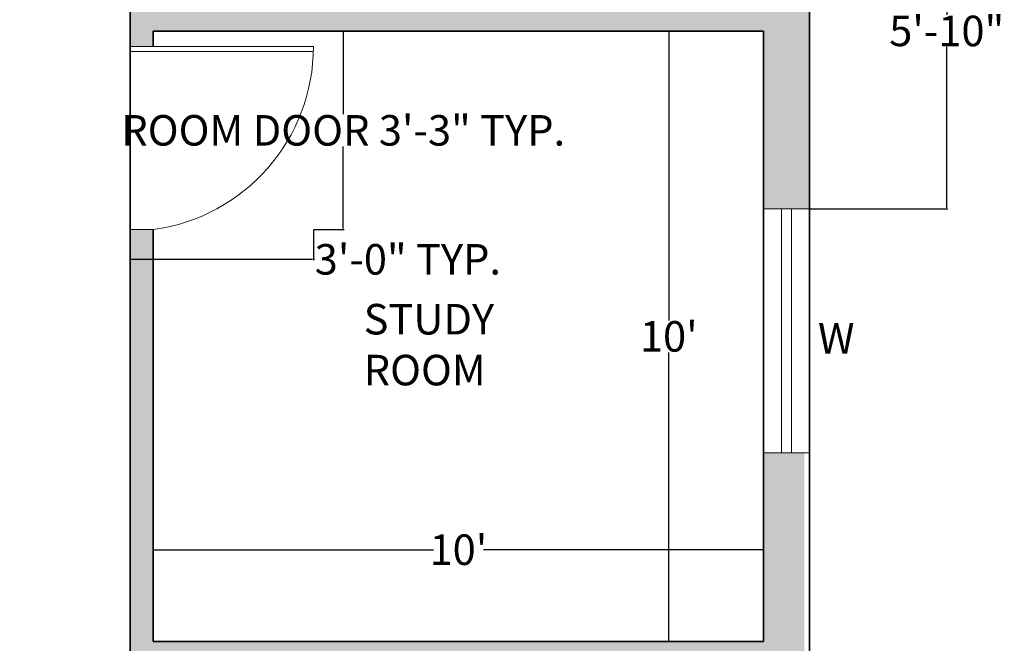
# Model space of a CAD drawing. Units: inches. Extents: x 302 to 1258, y 831 to 1373.
# Tile 11 of 13: x 1048 to 1241, y 1012 to 1135. Entities that reach past the tile are written whole.
import ezdxf

# ---------------------------------------------------------------- set-up
doc = ezdxf.new("R2010")
doc.units = ezdxf.units.IN
doc.header["$MEASUREMENT"] = 0
for name, color, linetype, lineweight in [('A-ANNO-DIMS', 2, 'Continuous', 18), ('A-ANNO-TEXT', 7, 'Continuous', 18), ('A-AREA-IDEN', 7, 'Continuous', 18), ('A-DOOR', 3, 'Continuous', 18), ('A-GLAZ', 4, 'Continuous', 18), ('A-WALL', 7, 'Continuous', 35), ('A-WALL-PATT', 251, 'Continuous', 13)]:
    doc.layers.add(name, color=color, linetype=linetype, lineweight=lineweight)
doc.styles.get("Standard").update_dxf_attribs({"font": 'arial.ttf'})
doc.dimstyles.get("Standard").update_dxf_attribs({"dimtxt": 6, "dimasz": 0.18, "dimexe": 0.18, "dimexo": 0.0625, "dimgap": 0.09, "dimtad": 0, "dimtih": 1, "dimtoh": 1, "dimdec": 1, "dimzin": 0, "dimdsep": 46, "dimlunit": 3, "dimtxsty": 'Standard', "dimcen": 0.09, "dimadec": 0, "dimazin": 0, "dimtfac": 1, "dimtdec": 1, "dimtofl": 0, "dimtmove": 0, "dimatfit": 3, "dimfxl": 1, "dimtolj": 1, "dimtzin": 0, "dimarcsym": 0})

# ---------------------------------------------------------------- blocks, each defined once
blk = doc.blocks.new('*D25')
at = {"layer": 'A-ANNO-DIMS', "color": 0, "lineweight": -2, "transparency": 16777216}
for p, q in [((1074.12, 1012.38), (1074.12, 1030.57)), ((1074.3, 1030.39), (1129.22, 1030.39)), ((1193.94, 1030.39), (1139.02, 1030.39)), ((1194.12, 1012.38), (1194.12, 1030.57))]:
    blk.add_line(p, q, dxfattribs=at)
at = {"layer": 'A-ANNO-DIMS', "color": 0, "transparency": 16777216}
for points in [[(1074.3, 1030.42), (1074.3, 1030.36), (1074.12, 1030.39)], [(1193.94, 1030.42), (1193.94, 1030.36), (1194.12, 1030.39)]]:
    blk.add_solid(points, dxfattribs=at)
at = {"layer": 'Defpoints', "color": 0, "transparency": 16777216}
for p in [(1194.12, 1030.39), (1074.12, 1012.32), (1194.12, 1012.32)]:
    blk.add_point(p, dxfattribs=at)
at = {"layer": 'A-ANNO-DIMS', "color": 0, "transparency": 16777216, "insert": (1134.12, 1030.39), "char_height": 6, "attachment_point": 5}
blk.add_mtext("\\A1;10'", dxfattribs=at)
blk = doc.blocks.new('*D26')
at = {"layer": 'A-ANNO-DIMS', "color": 0, "lineweight": -2, "transparency": 16777216}
for p, q in [((1194.06, 1132.32), (1175.3, 1132.32)), ((1175.48, 1132.14), (1175.48, 1075.47)), ((1175.48, 1012.5), (1175.48, 1069.17)), ((1194.06, 1012.32), (1175.3, 1012.32))]:
    blk.add_line(p, q, dxfattribs=at)
at = {"layer": 'A-ANNO-DIMS', "color": 0, "transparency": 16777216}
for points in [[(1175.45, 1132.14), (1175.51, 1132.14), (1175.48, 1132.32)], [(1175.45, 1012.5), (1175.51, 1012.5), (1175.48, 1012.32)]]:
    blk.add_solid(points, dxfattribs=at)
at = {"layer": 'Defpoints', "color": 0, "transparency": 16777216}
for p in [(1194.12, 1132.32), (1175.48, 1012.32), (1194.12, 1012.32)]:
    blk.add_point(p, dxfattribs=at)
at = {"layer": 'A-ANNO-DIMS', "color": 0, "transparency": 16777216, "insert": (1175.48, 1072.32), "char_height": 6, "attachment_point": 5}
blk.add_mtext("\\A1;10'", dxfattribs=at)
blk = doc.blocks.new('DOOR-36IN-ROOM')
for p, q in [((0, 39), (0, 36)), ((0, 36), (36, 36)), ((36, 36), (0, 36)), ((0, 36), (0, 0)), ((36, 35), (0, 35)), ((0, 0), (4.5, 0))]:
    blk.add_line(p, q)
blk.add_arc((-0.32, 36), 36.32, 277.6281, 0)
blk = doc.blocks.new('*D61')
at = {"layer": 'A-ANNO-DIMS', "color": 0, "lineweight": -2, "transparency": 16777216}
for p, q in [((1105.68, 1132.32), (1111.65, 1132.32)), ((1111.47, 1132.14), (1111.47, 1116.02)), ((1111.47, 1093.5), (1111.47, 1109.62)), ((1105.68, 1093.32), (1111.65, 1093.32))]:
    blk.add_line(p, q, dxfattribs=at)
at = {"layer": 'A-ANNO-DIMS', "color": 0, "transparency": 16777216}
for points in [[(1111.44, 1132.14), (1111.5, 1132.14), (1111.47, 1132.32)], [(1111.44, 1093.5), (1111.5, 1093.5), (1111.47, 1093.32)]]:
    blk.add_solid(points, dxfattribs=at)
at = {"layer": 'Defpoints', "color": 0, "transparency": 16777216}
for p in [(1105.62, 1132.32), (1111.47, 1132.32), (1105.62, 1093.32)]:
    blk.add_point(p, dxfattribs=at)
at = {"layer": 'A-ANNO-DIMS', "color": 0, "transparency": 16777216, "insert": (1111.47, 1112.82), "char_height": 6, "attachment_point": 5}
blk.add_mtext('\\A1;ROOM DOOR 3\'-3" TYP.', dxfattribs=at)
blk = doc.blocks.new('*D62')
at = {"layer": 'A-ANNO-DIMS', "color": 0, "lineweight": -2, "transparency": 16777216}
for p, q in [((1069.62, 1093.26), (1069.62, 1087.29)), ((1105.62, 1093.26), (1105.62, 1087.29)), ((1069.8, 1087.47), (1105.44, 1087.47)), ((1105.62, 1087.47), (1105.8, 1087.47))]:
    blk.add_line(p, q, dxfattribs=at)
at = {"layer": 'A-ANNO-DIMS', "color": 0, "transparency": 16777216}
for points in [[(1069.8, 1087.5), (1069.8, 1087.44), (1069.62, 1087.47)], [(1105.44, 1087.5), (1105.44, 1087.44), (1105.62, 1087.47)]]:
    blk.add_solid(points, dxfattribs=at)
at = {"layer": 'Defpoints', "color": 0, "transparency": 16777216}
for p in [(1069.62, 1093.32), (1105.62, 1093.32), (1105.62, 1087.47)]:
    blk.add_point(p, dxfattribs=at)
at = {"layer": 'A-ANNO-DIMS', "color": 0, "transparency": 16777216, "insert": (1124.18, 1087.47), "char_height": 6, "attachment_point": 5}
blk.add_mtext('\\A1;3\'-0" TYP.', dxfattribs=at)
blk = doc.blocks.new('*D93')
at = {"layer": 'A-ANNO-DIMS', "color": 0, "lineweight": -2, "transparency": 16777216}
for p, q in [((1203.18, 1167.3), (1230.3, 1167.3)), ((1230.12, 1167.12), (1230.12, 1135.51)), ((1230.12, 1097.6), (1230.12, 1129.21)), ((1203.18, 1097.42), (1230.3, 1097.42))]:
    blk.add_line(p, q, dxfattribs=at)
at = {"layer": 'A-ANNO-DIMS', "color": 0, "transparency": 16777216}
for points in [[(1230.09, 1167.12), (1230.15, 1167.12), (1230.12, 1167.3)], [(1230.09, 1097.6), (1230.15, 1097.6), (1230.12, 1097.42)]]:
    blk.add_solid(points, dxfattribs=at)
at = {"layer": 'Defpoints', "color": 0, "transparency": 16777216}
for p in [(1203.12, 1167.3), (1203.12, 1097.42), (1230.12, 1097.42)]:
    blk.add_point(p, dxfattribs=at)
at = {"layer": 'A-ANNO-DIMS', "color": 0, "transparency": 16777216, "insert": (1230.12, 1132.36), "char_height": 6, "attachment_point": 5}
blk.add_mtext('\\A1;5\'-10"', dxfattribs=at)

msp = doc.modelspace()

# ---------------------------------------------------------------- hatches: boundary and pattern name
at = {"layer": 'A-WALL-PATT'}
h = msp.add_hatch(color=256, dxfattribs=at)
h.dxf.hatch_style = 1
h.paths.add_polyline_path([(1203.12, 1254.71), (1194.12, 1254.71), (1194.12, 1213.32), (1087.12, 1213.32), (1087.12, 1208.82), (1093.62, 1208.82), (1093.62, 1205.82), (1098.12, 1205.82), (1098.12, 1208.82), (1194.12, 1208.82), (1194.12, 1191.3), (1203.12, 1191.3)])
h.paths.add_polyline_path([(1203.12, 1167.3), (1194.12, 1167.3), (1194.12, 1136.82), (1098.12, 1136.82), (1098.12, 1181.82), (1093.62, 1181.82), (1093.62, 1136.82), (1069.62, 1136.82), (1069.62, 1129.32), (1074.12, 1129.32), (1074.12, 1132.32), (1194.12, 1132.32), (1194.12, 1097.42), (1203.12, 1097.42)])
h = msp.add_hatch(color=256, dxfattribs=at)
h.dxf.hatch_style = 1
h.paths.add_polyline_path([(1074.12, 970.82), (1069.62, 970.82), (1069.62, 875.82), (855.12, 875.82), (855.12, 896.2), (846.12, 896.2), (846.12, 866.82), (1074.12, 866.82)])
h.paths.add_polyline_path([(1202.12, 1049.42), (1194.12, 1049.42), (1194.12, 1012.32), (1074.12, 1012.32), (1074.12, 1093.32), (1069.62, 1093.32), (1069.62, 1006.82), (1074.12, 1006.82), (1074.12, 1007.82), (1194.12, 1007.82), (1202.12, 1007.82)])

# ---------------------------------------------------------------- linework, layer by layer
at = {"layer": 'A-GLAZ'}
for p, q in [((1194.12, 1097.42), (1203.12, 1097.42)), ((1194.12, 1049.42), (1194.12, 1097.42)), ((1197.62, 1049.42), (1197.62, 1097.42)), ((1199.62, 1097.42), (1199.62, 1049.42)), ((1203.12, 1049.42), (1194.12, 1049.42))]:
    msp.add_line(p, q, dxfattribs=at)
at = {"layer": 'A-WALL'}
for p, q in [((1203.12, 866.82), (1203.12, 1342.32)), ((1069.62, 1136.82), (1069.62, 875.82)), ((1074.12, 1132.32), (1194.12, 1132.32)), ((1074.12, 1132.32), (1074.12, 1129.32)), ((1194.12, 1132.32), (1194.12, 1012.32)), ((1203.12, 1097.42), (1203.12, 866.82)), ((1074.12, 1093.32), (1074.12, 1012.32)), ((1074.12, 1012.32), (1194.12, 1012.32))]:
    msp.add_line(p, q, dxfattribs=at)

# ---------------------------------------------------------------- block references
at = {"layer": 'A-DOOR'}
msp.add_blockref('DOOR-36IN-ROOM', (1069.62, 1093.32), dxfattribs=at)

# ---------------------------------------------------------------- texts
at = {"layer": 'A-ANNO-TEXT', "insert": (1204.8, 1074.94), "char_height": 6, "attachment_point": 1}
msp.add_mtext_dynamic_manual_height_columns('W', width=16.4894, gutter_width=30, heights=[0], dxfattribs=at)
at = {"layer": 'A-AREA-IDEN', "insert": (1115.49, 1078.7), "char_height": 6, "attachment_point": 1}
msp.add_mtext_dynamic_manual_height_columns('STUDY\\PROOM', width=47.6227, gutter_width=30, heights=[0], dxfattribs=at)

# ---------------------------------------------------------------- dimensions: what is measured, and where the dimension line sits
at = {"layer": 'A-ANNO-DIMS'}
for base, p1, p2, override, picture, middle in [((1230.12, 1097.42), (1203.12, 1167.3), (1203.12, 1097.42), {"dimdec": 1, "dimlfac": 1, "dimrnd": 0, "dimzin": 1, "dimdsep": 46, "dimlunit": 4, "dimfrac": 2}, '*D93', (1230.12, 1132.36)), ((1175.48, 1012.32), (1194.12, 1132.32), (1194.12, 1012.32), {"dimclrd": 0, "dimclre": 0, "dimclrt": 0}, '*D26', (1175.48, 1072.32))]:
    dim = msp.add_linear_dim(base=base, p1=p1, p2=p2, angle=90, dimstyle='Standard', override=override, dxfattribs=at)
    dim.commit()
    dim.dimension.update_dxf_attribs({"geometry": picture, "text_midpoint": middle})
dim = msp.add_linear_dim(base=(1111.47, 1132.32), p1=(1105.62, 1093.32), p2=(1105.62, 1132.32), angle=90, text='ROOM DOOR <> TYP.', dimstyle='Standard', override={"dimdec": 1, "dimlfac": 1, "dimrnd": 0, "dimzin": 1, "dimdsep": 46, "dimlunit": 4, "dimfrac": 2}, dxfattribs=at)
dim.commit()
dim.dimension.update_dxf_attribs({"geometry": '*D61', "text_midpoint": (1111.47, 1112.82)})
dim = msp.add_linear_dim(base=(1105.62, 1087.47), p1=(1069.62, 1093.32), p2=(1105.62, 1093.32), text='<> TYP.', dimstyle='Standard', override={"dimdec": 1, "dimlfac": 1, "dimrnd": 0, "dimzin": 1, "dimdsep": 46, "dimlunit": 4, "dimfrac": 2}, dxfattribs=at)
dim.commit()
dim.dimension.update_dxf_attribs({"geometry": '*D62', "text_midpoint": (1124.18, 1087.47)})
dim = msp.add_linear_dim(base=(1194.12, 1030.39), p1=(1074.12, 1012.32), p2=(1194.12, 1012.32), dimstyle='Standard', override={"dimclrd": 0, "dimclre": 0, "dimclrt": 0}, dxfattribs=at)
dim.commit()
dim.dimension.update_dxf_attribs({"geometry": '*D25', "text_midpoint": (1134.12, 1030.39)})

doc.saveas('drawing.dxf')
